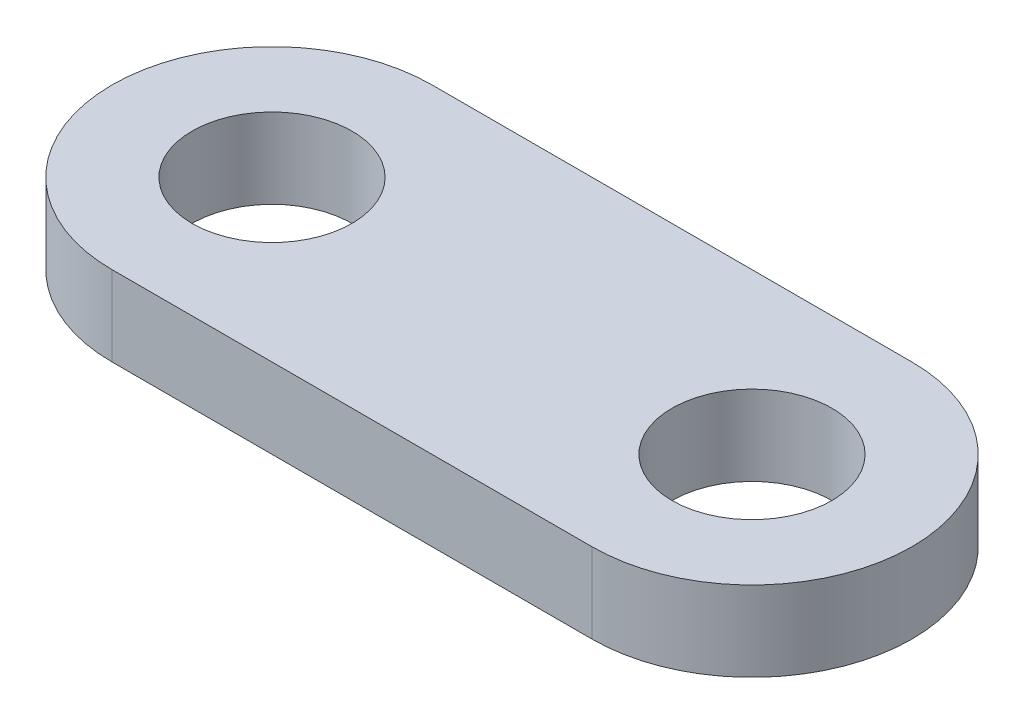
from build123d import *

# Parameters (mm, degrees)
LINK_PROFILE_R       = 5
LINK_PLATE_5MM_DEPTH = 5


with BuildPart() as part:
    # Link Profile → Link Plate 5mm (new body)
    with BuildSketch(Plane(origin=(0, 0, 0), x_dir=(1, 0, 0), z_dir=(0, 1, 0))):
        with BuildLine():
            Line((-15, 10), (15, 10))
            ThreePointArc((15, 10), (25, 0), (15, -10))
            Line((15, -10), (-15, -10))
            ThreePointArc((-15, -10), (-25, 0), (-15, 10))
        make_face()
        with Locations(Location((-15, 0, 0), (0, 0, 270))):
            Circle(LINK_PROFILE_R, mode=Mode.SUBTRACT)
        with Locations(Location((15, 0, 0), (0, 0, 270))):
            Circle(LINK_PROFILE_R, mode=Mode.SUBTRACT)
    extrude(amount=LINK_PLATE_5MM_DEPTH)


solid = part.part
